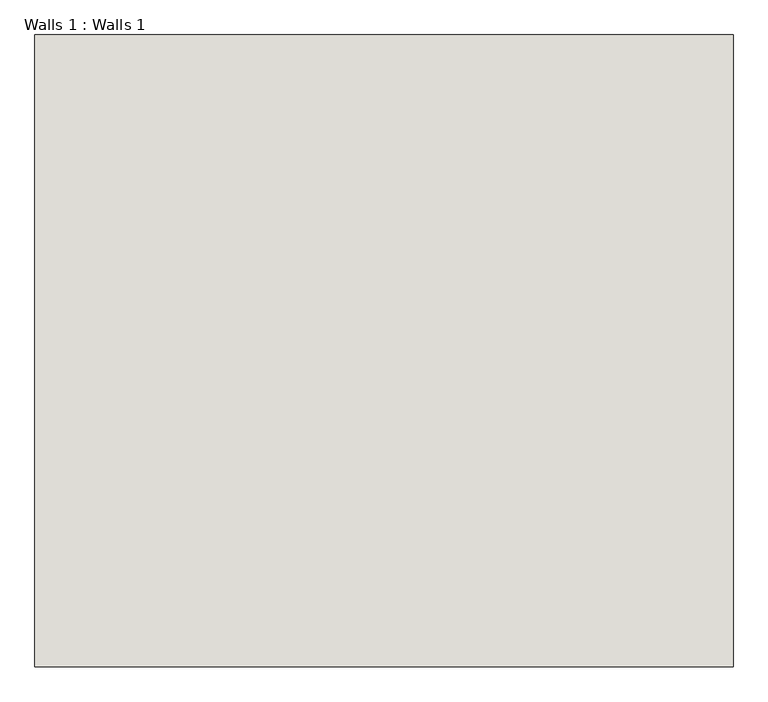
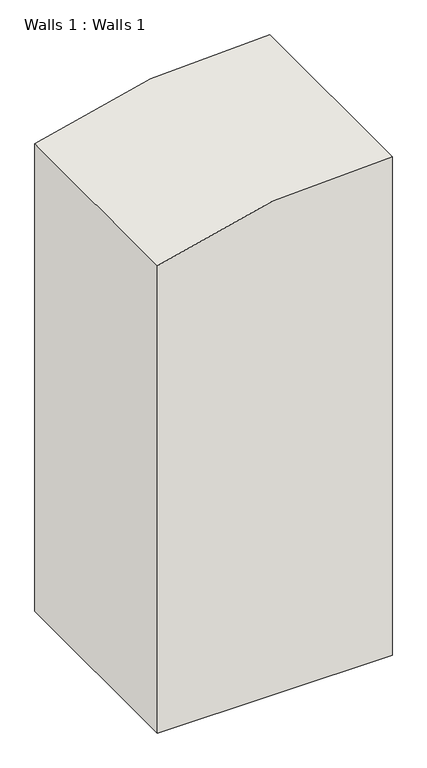
"""IFC4 building model written with IfcOpenShell, lengths in millimetres: wall geometry, Walls 1 : Walls 1."""

from ifc_helpers import new_model, si_unit, point, frame, frame_2d, origin, place, context, project, spatial, polyline, circle_curve, trimmed, segment, composite_curve, outline, extrude, source, transform, mapped, element, save


def walls_1_walls_1_63333409(model_context):
    return source(origin(), model_context, "Body", "SweptSolid", [
        extrude(outline(composite_curve([segment(polyline([(20030.620294, -18502.079547), (-400.0, -18502.079547), (-400.0, -8802.079547), (21400.0, -8802.079547)]), True, "CONTINUOUS"), segment(trimmed(circle_curve(frame_2d((-3469.7681279, -10237.7954874)), 24911.1751428), [point((21400.0, -8802.079547))], [point((20030.620294, -18502.079547))], False, "CARTESIAN"), True, "CONTINUOUS")], self_intersect=False)), frame((0.0, -10393.2199515, 0.0), z_axis=(0.0, 1.0, 0.0), x_axis=(0.0, 0.0, 1.0)), (0.0, 0.0, 1.0), 8776.8191547),
    ])


if __name__ == "__main__":
    model = new_model("IFC4")
    model_context = context("Model", 3, world=origin())
    ifc_project = project(units=[si_unit("LENGTHUNIT", "METRE", prefix="MILLI")], contexts=[model_context])
    site = spatial("IfcSite", under=ifc_project)
    building = spatial("IfcBuilding", under=site)
    placement = place(None, origin())
    walls_1_walls_1_shape = walls_1_walls_1_63333409(model_context)
    element("IfcWall", 1, ObjectType="Walls 1 : Walls 1", at=placement, inside=building, context=model_context, shape_type="MappedRepresentation", body=[
        mapped(walls_1_walls_1_shape, transform((0.0, 0.0, 0.0), x_axis=(1.0, 0.0, 0.0), y_axis=(0.0, 1.0, 0.0), z_axis=(0.0, 0.0, 1.0))),
    ])
    save(model, "model.ifc")

# Revit data of these elements
# Element 1 (IfcWall, "Walls 1 : Walls 1")
#   Materials on its faces: "Default Wall"
# Materials
#   "Default Wall": colour RGB 80 80 80, transparency 0
